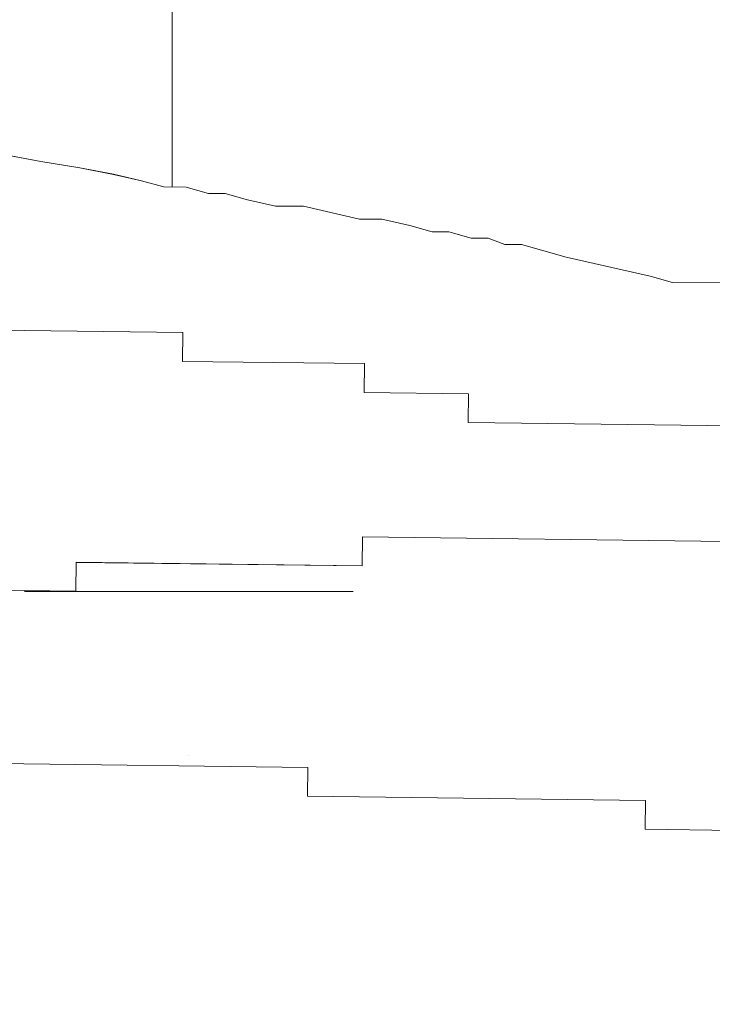
# Model space of a CAD drawing. Units: inches. Extents: x -466983 to 1020, y 324 to 318697.
# Tile 81 of 97: x 656.235 to 659.546, y 944.006 to 948.713. Entities that reach past the tile are written whole.
import ezdxf

# ---------------------------------------------------------------- set-up
doc = ezdxf.new("R2010")
doc.units = ezdxf.units.IN
doc.header["$MEASUREMENT"] = 0
doc.layers.add('A-FLOR-PATT', color=252, linetype='Continuous', lineweight=13)
doc.layers.add('A-FURN', color=8, linetype='Continuous', lineweight=18)

# ---------------------------------------------------------------- blocks, each defined once
blk = doc.blocks.new('L Shaped Sofa')
at = {"ltscale": 2}
for p, q in [((2389.455, 739.834), (2390.5892, 739.8201)), ((2390.5892, 739.8201), (2390.5861, 739.5682)), ((2390.5861, 739.5682), (2393.535, 739.5322)), ((2393.535, 739.5322), (2393.5319, 739.2803)), ((2393.5319, 739.2803), (2396.4808, 739.2443)), ((2394.5686, 739.1785), (2394.5686, 739.1785)), ((2396.0014, 737.7457), (2393.1358, 737.7457)), ((2395.5519, 737.492), (2395.555, 737.7439)), ((2395.555, 737.7439), (2399.8649, 737.6912)), ((2393.0536, 737.2705), (2393.0567, 737.5224)), ((2393.0567, 737.5224), (2395.5519, 737.492)), ((2389.8779, 737.3093), (2393.0536, 737.2705)), ((2386.9167, 736.3377), (2392.134, 736.274)), ((2392.134, 736.274), (2392.1309, 736.0221)), ((2392.1309, 736.0221), (2393.0382, 736.011)), ((2393.0382, 736.011), (2393.0352, 735.7591)), ((2393.0352, 735.7591), (2394.623, 735.7397)), ((2394.623, 735.7397), (2394.6199, 735.4878)), ((2394.6199, 735.4878), (2397.1151, 735.4573)), ((2387.7166, 735.0656), (2390.3515, 735.0532)), ((2390.3515, 735.0532), (2390.5464, 734.9981)), ((2390.5464, 734.9981), (2391.2773, 734.832)), ((2391.2773, 734.832), (2391.667, 734.7217)), ((2391.667, 734.7217), (2391.8134, 734.7211)), ((2391.8134, 734.7211), (2391.9595, 734.6662)), ((2391.9595, 734.6662), (2392.1058, 734.6655)), ((2392.1058, 734.6655), (2392.3007, 734.6103)), ((2392.3007, 734.6103), (2392.4471, 734.6096)), ((2392.4471, 734.6096), (2392.6419, 734.5545)), ((2392.6419, 734.5545), (2392.8856, 734.4992)), ((2392.8856, 734.4992), (2393.0807, 734.4982)), ((2393.0807, 734.4982), (2393.568, 734.3875)), ((2393.568, 734.3875), (2393.812, 734.3864)), ((2393.812, 734.3864), (2394.0556, 734.331)), ((2394.0556, 734.331), (2394.2505, 734.2759)), ((2394.2505, 734.2759), (2394.3969, 734.2752)), ((2394.3969, 734.2752), (2394.5917, 734.2201)), ((2394.5917, 734.2201), (2394.7869, 734.2191)), ((2394.7123, 728.35), (2394.7123, 734.2195)), ((2394.7869, 734.2191), (2394.9818, 734.164)), ((2394.9818, 734.164), (2395.2254, 734.1087)), ((2395.2254, 734.1087), (2395.5178, 734.0531)), ((2395.5178, 734.0531), (2395.8591, 733.9972)), ((2395.8591, 733.9972), (2396.444, 733.8861))]:
    blk.add_line(p, q, dxfattribs=at)

msp = doc.modelspace()

# ---------------------------------------------------------------- hatches: boundary and pattern name
at = {"layer": 'A-FLOR-PATT', "transparency": 33554572}
h = msp.add_hatch(dxfattribs=at)
h.set_pattern_fill('ANSI37', color=256, scale=30)
h.set_pattern_definition([(45, (-1212.4137, -290.035), (-2.6516504, 2.6516504), []), (135, (-1212.4137, -290.035), (-2.6516504, -2.6516504), [])])
h.paths.add_polyline_path([(901.8057, 1075.9377), (900.6144, 1075.9377), (900.6144, 1065.3856), (899.391, 1065.3856), (898.0911, 1065.3856), (892.8356, 1058.7098, -0.258377), (892.1875, 1058.3509), (879.9848, 1058.3509, -0.20177), (879.4382, 1058.5808), (874.0812, 1065.3856), (872.7813, 1065.3856), (871.5579, 1065.3856), (871.5579, 1075.9377), (813.8057, 1075.9377), (813.8057, 1044.7922), (832.3947, 1044.7922, -0.394795), (848.6602, 1028.5356), (848.6602, 1009.9377), (901.8057, 1009.9377), (901.8057, 1015.9377), (901.3057, 1015.9377), (871.3057, 1015.9377), (871.3057, 1017.2502), (871.3344, 1017.2502, -0.401453), (901.3057, 1045.9377), (901.8057, 1045.9377)])
edge = h.paths.add_edge_path(flags=16)
edge.add_line((847.7731, 1068.9486), (847.7731, 1073.7088))
edge.add_arc((849.2269, 1073.7088), 1.4538, 90, 180, ccw=False)
edge.add_line((849.2269, 1075.1627), (864.4921, 1075.1627))
edge.add_arc((864.4921, 1073.7088), 1.4538, 0, 90, ccw=False)
edge.add_line((865.9459, 1073.7088), (865.9459, 1069.0035))
edge.add_arc((832.6447, 1068.9761), 33.3012, -20.61234, 0.04725, ccw=False)
edge.add_ellipse((856.8595, 1058.48), major_axis=(0, 10.2131), ratio=0.6859192, start_angle=100.00884, end_angle=259.99116, ccw=False)
edge.add_arc((881.0742, 1068.9761), 33.3012, 180.04725, 200.61234, ccw=False)
h.paths.add_polyline_path([(853.1456, 1066.4815), (853.1456, 1066.4534), (853.1463, 1066.4534, 0.433107), (852.9166, 1066.6849), (852.9166, 1066.4534), (853.1456, 1066.4534), (853.1456, 1066.4815), (853.088, 1066.6122, 0.697939), (852.6995, 1066.4534), (852.7003, 1066.4534), (852.7003, 1066.4815), (852.9166, 1067.0012), (852.9166, 1066.6849, -0.396254)], flags=0)
h.paths.add_polyline_path([(861.0187, 1066.4815), (861.0187, 1066.4534), (861.0194, 1066.4534, 0.416404), (860.8024, 1066.6849), (860.8024, 1066.4534), (861.0187, 1066.4534), (861.0187, 1066.4815), (860.9672, 1066.6053, 0.713344), (860.5726, 1066.4534), (860.5734, 1066.4534), (860.5734, 1066.4815), (860.8024, 1067.0012), (860.8024, 1066.6849, -0.379973)], flags=0)
edge = h.paths.add_edge_path(flags=0)
edge.add_spline(control_points=[(861.1298, 1065.7855), (861.4661, 1065.2478), (861.6134, 1065.0161), (861.9833, 1064.3736), (862.1924, 1063.9443), (862.5614, 1063.0391), (862.7212, 1062.5633), (862.9865, 1061.5781), (863.092, 1061.0689), (863.2452, 1060.031), (863.293, 1059.5025), (863.3295, 1058.4409), (863.3181, 1057.9078), (863.2366, 1056.8518), (863.1664, 1056.3289), (862.9695, 1055.308), (862.8427, 1054.8099), (862.5365, 1053.8522), (862.3571, 1053.3927), (861.9514, 1052.5249), (861.7251, 1052.1166), (861.233, 1051.3622), (860.9672, 1051.0162), (860.4048, 1050.3949), (860.1082, 1050.1197), (859.4937, 1049.6461), (859.1758, 1049.4476), (858.5276, 1049.1299), (858.1973, 1049.0107), (857.5315, 1048.8518), (857.1959, 1048.8121), (856.5249, 1048.812), (856.1894, 1048.8515), (855.5236, 1049.0101), (855.1933, 1049.1291), (854.545, 1049.4465), (854.2271, 1049.6449), (853.6124, 1050.1183), (853.3158, 1050.3933), (852.7533, 1051.0143), (852.4874, 1051.3602), (851.9952, 1052.1144), (851.7688, 1052.5225), (851.3629, 1053.3902), (851.1834, 1053.8496), (850.877, 1054.8071), (850.7501, 1055.3051), (850.553, 1056.326), (850.4827, 1056.8488), (850.401, 1057.9048), (850.3895, 1058.4379), (850.4257, 1059.4995), (850.4734, 1060.0281), (850.6265, 1061.066), (850.7318, 1061.5753), (850.9969, 1062.5605), (851.1567, 1063.0365), (851.5254, 1063.9418), (851.7345, 1064.3712), (852.1056, 1065.0164), (852.2544, 1065.2503), (852.6082, 1065.7335)], knot_values=[3.915332, 3.915332, 3.915332, 3.915332, 4.013468, 4.013468, 4.175532, 4.175532, 4.337596, 4.337596, 4.49966, 4.49966, 4.661724, 4.661724, 4.823788, 4.823788, 4.985852, 4.985852, 5.147916, 5.147916, 5.30998, 5.30998, 5.472044, 5.472044, 5.634109, 5.634109, 5.796173, 5.796173, 5.958237, 5.958237, 6.120301, 6.120301, 6.282365, 6.282365, 6.444429, 6.444429, 6.606493, 6.606493, 6.768557, 6.768557, 6.930621, 6.930621, 7.092685, 7.092685, 7.254749, 7.254749, 7.416813, 7.416813, 7.578878, 7.578878, 7.740942, 7.740942, 7.903006, 7.903006, 8.06507, 8.06507, 8.227134, 8.227134, 8.389198, 8.389198, 8.551262, 8.551262, 8.65037, 8.65037, 8.65037, 8.65037], degree=3, periodic=0)
edge.add_line((852.6421, 1065.7855), (861.1298, 1065.7855))
edge = h.paths.add_edge_path(flags=0)
edge.add_ellipse((856.8496, 1057.7432), major_axis=(0, 7.7921), ratio=0.687861, start_angle=0, end_angle=360)
h.paths.add_polyline_path([(848.8634, 1069.3891), (848.8634, 1073.9605, -0.414214), (849.9538, 1075.0508), (863.7652, 1075.0508, -0.414214), (864.8555, 1073.9605), (864.8555, 1069.3891, -0.388936), (864.5237, 1069.027, -0.043561), (849.1953, 1069.027, -0.388936)], flags=0)
h.paths.add_polyline_path([(853.1006, 1068.1122, -1), (852.6775, 1068.1122, -1)], flags=0)
edge = h.paths.add_edge_path(flags=0)
edge.add_ellipse((856.8595, 1057.3378), major_axis=(0, 2.207), ratio=0.657164, start_angle=0, end_angle=360)
h.paths.add_polyline_path([(861.0415, 1068.1122, -1), (860.6184, 1068.1122, -1)], flags=0)
edge = h.paths.add_edge_path()
edge.add_line((573.9537, 1057.3412), (573.9537, 1075.9377))
edge.add_line((573.9537, 1075.9377), (558.7308, 1075.9377))
edge.add_line((558.7308, 1075.9377), (558.7308, 1065.3856))
edge.add_line((558.7308, 1065.3856), (557.5074, 1065.3856))
edge.add_line((557.5074, 1065.3856), (556.2075, 1065.3856))
edge.add_line((556.2075, 1065.3856), (550.952, 1058.7098))
edge.add_arc((550.3039, 1059.1155), 0.7646, 270, 327.9483, ccw=False)
edge.add_line((550.3039, 1058.3509), (538.1012, 1058.3509))
edge.add_arc((538.1012, 1059.1155), 0.7646, 224.3704, 270, ccw=False)
edge.add_line((537.5546, 1058.5808), (532.1976, 1065.3856))
edge.add_line((532.1976, 1065.3856), (530.8977, 1065.3856))
edge.add_line((530.8977, 1065.3856), (529.6743, 1065.3856))
edge.add_line((529.6743, 1065.3856), (529.6743, 1075.9377))
edge.add_line((529.6743, 1075.9377), (520.8057, 1075.9377))
edge.add_line((520.8057, 1075.9377), (520.8057, 1045.9377))
edge.add_line((520.8057, 1045.9377), (521.3057, 1045.9377))
edge.add_arc((521.3057, 1015.9377), 30, 2.50749, 90, ccw=False)
edge.add_line((551.277, 1017.2502), (551.3057, 1017.2502))
edge.add_line((551.3057, 1017.2502), (551.3057, 1015.9377))
edge.add_line((551.3057, 1015.9377), (520.8057, 1015.9377))
edge.add_line((520.8057, 1015.9377), (520.8057, 1009.9377))
edge.add_line((520.8057, 1009.9377), (559.1913, 1010.4022))
edge.add_arc((559.1913, 1011.856), 1.4538, 180, 270, ccw=False)
edge.add_line((557.7375, 1011.856), (557.7375, 1016.5613))
edge.add_arc((591.0386, 1016.5888), 33.3012, 159.38766, 180.04725, ccw=False)
edge.add_ellipse((566.8239, 1027.0848), major_axis=(0, 10.2131), ratio=0.6859192, start_angle=280.00884, end_angle=439.99116, ccw=False)
edge.add_arc((542.6091, 1016.5888), 33.3012, 0.04725, 20.61234, ccw=False)
edge.add_line((575.9103, 1016.6162), (575.9103, 1011.856))
edge.add_arc((574.4565, 1011.856), 1.4538, -90, 0, ccw=False)
edge.add_line((574.4565, 1010.4022), (608.8057, 1009.9377))
edge.add_line((608.8057, 1009.9377), (608.8057, 1041.0857))
edge.add_line((608.8057, 1041.0857), (590.2179, 1041.0857))
edge.add_arc((590.775, 1057.9074), 16.8309, 181.92775, 268.10321, ccw=False)
edge = h.paths.add_edge_path()
edge.add_ellipse((494.2443, 583.6204), major_axis=(0, 10.2131), ratio=0.6859192, start_angle=280.00884, end_angle=439.99116, ccw=False)
edge.add_arc((470.0296, 573.1243), 33.3012, 0.04725, 20.61234, ccw=False)
edge.add_line((503.3307, 573.1518), (503.3307, 568.3916))
edge.add_arc((501.8769, 568.3916), 1.4538, -90, 0, ccw=False)
edge.add_line((501.8769, 566.9377), (539.8057, 566.9377))
edge.add_line((539.8057, 566.9377), (539.8057, 572.9377))
edge.add_line((539.8057, 572.9377), (539.3057, 572.9377))
edge.add_line((539.3057, 572.9377), (509.3057, 572.9377))
edge.add_line((509.3057, 572.9377), (509.3057, 574.2502))
edge.add_line((509.3057, 574.2502), (509.3344, 574.2502))
edge.add_arc((539.3057, 572.9377), 30, 90, 177.49251, ccw=False)
edge.add_line((539.3057, 602.9377), (539.8057, 602.9377))
edge.add_line((539.8057, 602.9377), (539.8057, 626.9377))
edge.add_line((539.8057, 626.9377), (531.7718, 626.9377))
edge.add_line((531.7718, 626.9377), (531.7718, 616.3856))
edge.add_line((531.7718, 616.3856), (530.5484, 616.3856))
edge.add_line((530.5484, 616.3856), (529.2485, 616.3856))
edge.add_line((529.2485, 616.3856), (523.7105, 609.3509))
edge.add_line((523.7105, 609.3509), (510.7766, 609.3509))
edge.add_line((510.7766, 609.3509), (505.2386, 616.3856))
edge.add_line((505.2386, 616.3856), (503.9387, 616.3856))
edge.add_line((503.9387, 616.3856), (502.7153, 616.3856))
edge.add_line((502.7153, 616.3856), (502.7153, 626.9377))
edge.add_line((502.7153, 626.9377), (481.6983, 626.9377))
edge.add_line((481.6983, 626.9377), (481.6983, 610.995))
edge.add_arc((467.2703, 611.4728), 14.4359, 271.92775, 358.10321, ccw=False)
edge.add_line((467.7559, 597.0451), (451.8057, 597.0451))
edge.add_line((451.8057, 597.0451), (451.8057, 584.4035))
edge.add_line((451.8057, 584.4035), (451.8057, 566.9377))
edge.add_line((451.8057, 566.9377), (486.6117, 566.9377))
edge.add_arc((486.6117, 568.3916), 1.4538, 180, 270, ccw=False)
edge.add_line((485.1579, 568.3916), (485.1579, 573.0969))
edge.add_arc((518.4591, 573.1243), 33.3012, 159.38766, 180.04725, ccw=False)
h.paths.add_polyline_path([(836.2609, 1020.7328), (879.8898, 1020.7328), (879.8898, 1039.3902), (836.2609, 1039.3902)], flags=25)
h.paths.add_polyline_path([(549.9851, 1036.7492), (593.614, 1036.7492), (593.614, 1055.4065), (549.9851, 1055.4065)], flags=24)
h.paths.add_polyline_path([(475.123, 595.5959), (518.752, 595.5959), (518.752, 614.2532), (475.123, 614.2532)], flags=24)
h = msp.add_hatch(dxfattribs=at)
h.set_pattern_fill('ANSI37', color=256, scale=20)
h.set_pattern_definition([(45, (-1212.4137, -290.035), (-1.767767, 1.767767), []), (135, (-1212.4137, -290.035), (-1.767767, -1.767767), [])])
h.paths.add_polyline_path([(809.8057, 870.9377), (809.8057, 888.1519), (806.9985, 888.1519), (802.6624, 888.1519), (789.3832, 888.1519), (786.2846, 888.1519, -0.414214), (785.4991, 888.9374), (785.4991, 900.1959), (785.4991, 908.4696, -0.414214), (786.8082, 909.7787, -0.414214), (785.4991, 911.0878), (785.4991, 929.1015, -0.414214), (786.8082, 930.4106, -0.414214), (785.4991, 931.7197), (785.4991, 931.9039, -0.414214), (784.19, 930.5948), (766.7223, 930.5948, -0.412359), (765.4132, 931.8956, -0.413741), (764.1145, 930.5782), (744.5781, 930.422, -0.416556), (743.7864, 931.2075), (743.7864, 933.5153), (742.2154, 933.5153), (742.2154, 952.024, -0.001344), (743.7864, 952.1998), (743.7864, 953.9377), (678.5915, 953.9377), (678.5915, 951.1305), (678.5915, 946.7945), (678.5915, 933.5153), (678.5915, 930.4166, -0.414214), (677.806, 929.6312), (666.5475, 929.6312), (658.2738, 929.6312, -0.414214), (656.9647, 930.9403, -0.414214), (655.6556, 929.6312), (637.6419, 929.6312, -0.414214), (636.3328, 930.9403, -0.414214), (635.0237, 929.6312), (634.8395, 929.6312, -0.414214), (636.1486, 928.322), (636.1486, 910.8544, -0.412359), (634.8478, 909.5452, -0.413741), (636.1653, 908.2466), (636.3214, 888.7102, -0.416556), (635.5359, 887.9184), (633.2281, 887.9184), (633.2281, 886.3475), (614.7194, 886.3475, -0.001344), (614.5436, 887.9184), (612.8057, 887.9184), (612.8057, 834.9377), (612.8057, 752.9377), (612.8057, 748.9377), (612.8057, 697.9377), (654.8057, 697.9377), (654.8057, 701.9377), (715.8057, 701.9377), (715.8057, 737.4353), (774.2918, 737.4353), (774.2918, 795.9377), (809.8057, 795.9377)])
h.paths.add_polyline_path([(679.2761, 849.5757, 0.102523), (682.1475, 849.2608, -0.080461), (694.5428, 849.7725, -0.283899), (694.4822, 849.0082, 0.136605), (694.4068, 848.8103, -0.030441), (694.5428, 846.8929), (694.5428, 842.6198), (694.5428, 838.3466, -0.028219), (694.4246, 836.5684), (694.425, 836.5684, 0.196187), (694.4456, 836.2708, -0.302897), (694.5428, 835.467, -0.080461), (682.1475, 835.9787, 0.102523), (679.2761, 835.6638, -0.58611), (678.6457, 836.0169), (678.6457, 849.2227, -0.58611)], flags=16)
h.paths.add_polyline_path([(679.5173, 848.6515, 0.699597), (679.476, 848.6342, 1.20716), (679.1935, 848.7422, 0.010621)], flags=0)
h.paths.add_polyline_path([(679.4923, 836.5608, -0.013798), (679.9178, 836.6594, -0.071703), (682.8533, 837.1434, -0.165743), (682.1665, 839.1006), (682.1665, 842.6094), (682.1665, 846.0603, -0.240616), (683.4733, 848.6767, -0.068263), (693.9295, 849.0082), (693.7875, 848.7083), (693.7875, 849.0228, 0.067332), (683.4733, 848.6767, 0.240616), (682.1665, 846.0603), (682.1665, 842.6094), (682.1665, 839.1006, 0.23459), (683.461, 836.5513, 0.068093), (693.7875, 836.1955), (693.7875, 836.5104), (693.9296, 836.2102, -0.077215), (682.2421, 836.7815, 0.086627), (679.5283, 836.5701, -0.628402), (679.5029, 836.5735), (679.5029, 836.6071, 0.910458)], flags=0)
h.paths.add_polyline_path([(679.476, 848.6364), (679.2069, 848.647), (679.2069, 836.5718, 0.913566), (679.3645, 836.5861), (679.476, 836.5824)], flags=0)
h.paths.add_polyline_path([(679.2761, 829.8604, 0.102523), (682.1475, 829.5455, -0.080461), (694.5428, 830.0572, -0.283899), (694.4822, 829.2929, 0.136605), (694.4068, 829.095, -0.030441), (694.5428, 827.1776), (694.5428, 822.9045), (694.5428, 818.6314, -0.028219), (694.4246, 816.8531), (694.425, 816.8532, 0.196187), (694.4456, 816.5555, -0.302897), (694.5428, 815.7517, -0.080461), (682.1475, 816.2635, 0.102523), (679.2761, 815.9485, -0.58611), (678.6457, 816.3016), (678.6457, 829.5074, -0.58611)], flags=16)
h.paths.add_polyline_path([(679.5173, 828.9362, 0.699597), (679.476, 828.9189, 1.20716), (679.1935, 829.0269, 0.010621)], flags=0)
h.paths.add_polyline_path([(679.4923, 816.8456, -0.013798), (679.9178, 816.9441, -0.071703), (682.8533, 817.4281, -0.165743), (682.1665, 819.3853), (682.1665, 822.8941), (682.1665, 826.345, -0.240616), (683.4733, 828.9614, -0.068263), (693.9295, 829.2929), (693.7875, 828.9931), (693.7875, 829.3076, 0.067332), (683.4733, 828.9614, 0.240616), (682.1665, 826.345), (682.1665, 822.8941), (682.1665, 819.3853, 0.23459), (683.461, 816.836, 0.068093), (693.7875, 816.4802), (693.7875, 816.7952), (693.9296, 816.4949, -0.077215), (682.2421, 817.0662, 0.086627), (679.5283, 816.8549, -0.628402), (679.5029, 816.8582), (679.5029, 816.8918, 0.910458)], flags=0)
h.paths.add_polyline_path([(679.476, 828.9211), (679.2069, 828.9317), (679.2069, 816.8565, 0.913566), (679.3645, 816.8708), (679.476, 816.8671)], flags=0)
h.paths.add_polyline_path([(679.2761, 810.1451, 0.102523), (682.1475, 809.8302, -0.080461), (694.5428, 810.342, -0.3023), (694.4466, 809.5394, 0.10023), (694.4058, 809.3878, -0.03057), (694.5428, 807.4623), (694.5428, 803.1892), (694.5428, 798.9161, -0.03057), (694.4058, 796.9906, 0.10023), (694.4466, 796.839, -0.3023), (694.5428, 796.0365, -0.080461), (682.1475, 796.5482, 0.102523), (679.2761, 796.2333, -0.58611), (678.6457, 796.5863), (678.6457, 809.7921, -0.58611)], flags=16)
h.paths.add_polyline_path([(679.5173, 809.2417, 0.699597), (679.476, 809.2244, 1.20716), (679.1935, 809.3324, 0.010621)], flags=0)
h.paths.add_polyline_path([(679.4923, 797.151, -0.013798), (679.9178, 797.2496, -0.071703), (682.8533, 797.7336, -0.165743), (682.1665, 799.6908), (682.1665, 803.1996), (682.1665, 806.6505, -0.239349), (683.461, 809.2577, -0.072465), (694.4468, 809.5405, 0.197932), (694.425, 809.2405), (693.7875, 809.2985), (693.7875, 809.6135, 0.068093), (683.461, 809.2577, 0.239349), (682.1665, 806.6505), (682.1665, 803.1996), (682.1665, 799.6908, 0.235854), (683.4733, 797.1323, 0.067332), (693.7875, 796.7861), (693.7875, 797.1006), (694.425, 797.1586, 0.197932), (694.4468, 796.8586, -0.080419), (682.1557, 797.3795, 0.083867), (679.5283, 797.1603, -0.628402), (679.5029, 797.1637), (679.5029, 797.1973, 0.910458)], flags=0)
h.paths.add_polyline_path([(679.2069, 809.2372), (679.2069, 797.162, 0.913566), (679.3645, 797.1763), (679.476, 797.1726), (679.476, 809.2266)], flags=0)
h.paths.add_polyline_path([(695.3643, 853.2989), (728.2231, 853.2989), (728.2231, 771.1519), (695.3643, 771.1519)], flags=16)
h.paths.add_polyline_path([(696.0215, 852.6417), (727.5659, 852.6417), (727.5659, 771.809), (696.0215, 771.809)], flags=0)
h.paths.add_polyline_path([(679.2761, 788.7869, 0.102523), (682.1475, 788.472, -0.080461), (694.5428, 788.9837, -0.3023), (694.4466, 788.1812, 0.10023), (694.4058, 788.0296, -0.03057), (694.5428, 786.1041), (694.5428, 781.831), (694.5428, 777.5578, -0.03057), (694.4058, 775.6323, 0.10023), (694.4466, 775.4808, -0.3023), (694.5428, 774.6782, -0.080461), (682.1475, 775.19, 0.102523), (679.2761, 774.875, -0.58611), (678.6457, 775.2281), (678.6457, 788.4339, -0.58611)], flags=16)
h.paths.add_polyline_path([(679.5173, 787.8834, 0.699597), (679.476, 787.8662, 1.20716), (679.1935, 787.9742, 0.010621)], flags=0)
h.paths.add_polyline_path([(679.4923, 775.7928, -0.013798), (679.9178, 775.8914, -0.071703), (682.8533, 776.3753, -0.165743), (682.1665, 778.3325), (682.1665, 781.8414), (682.1665, 785.2922, -0.239349), (683.461, 787.8995, -0.072465), (694.4468, 788.1823, 0.197932), (694.425, 787.8823), (693.7875, 787.9403), (693.7875, 788.2553, 0.068093), (683.461, 787.8995, 0.239349), (682.1665, 785.2922), (682.1665, 781.8414), (682.1665, 778.3325, 0.235854), (683.4733, 775.7741, 0.067332), (693.7875, 775.4279), (693.7875, 775.7424), (694.425, 775.8004, 0.197932), (694.4468, 775.5004, -0.080419), (682.1557, 776.0212, 0.083867), (679.5283, 775.8021, -0.628402), (679.5029, 775.8054), (679.5029, 775.8391, 0.910458)], flags=0)
h.paths.add_polyline_path([(679.2069, 787.8789), (679.2069, 775.8038, 0.913566), (679.3645, 775.818), (679.476, 775.8144), (679.476, 787.8684)], flags=0)
h.paths.add_polyline_path([(704.641, 854.1204, -0.080461), (705.1527, 866.5157, 0.102523), (704.8378, 869.3871, -0.58611), (705.1908, 870.0174), (718.3966, 870.0174, -0.58611), (718.7496, 869.3871, 0.102523), (718.4347, 866.5157, -0.080461), (718.9465, 854.1204, -0.3023), (718.1439, 854.2166, 0.10023), (717.9924, 854.2574, -0.03057), (716.0668, 854.1204), (711.7937, 854.1204), (707.5206, 854.1204, -0.03057), (705.5951, 854.2574, 0.10023), (705.4435, 854.2166, -0.3023)], flags=16)
h.paths.add_polyline_path([(717.8462, 869.1459, 0.699597), (717.8289, 869.1872, 1.20716), (717.9369, 869.4697, 0.010621)], flags=0)
h.paths.add_polyline_path([(705.4631, 854.2164, -0.080419), (705.984, 866.5074, 0.083867), (705.7648, 869.1349, -0.628402), (705.7682, 869.1603), (705.8018, 869.1603, 0.910458), (705.7555, 869.1709, -0.013798), (705.8541, 868.7454, -0.071703), (706.3381, 865.8099, -0.165743), (708.2953, 866.4967), (711.8041, 866.4967), (715.255, 866.4967, -0.239349), (717.8622, 865.2022, -0.072465), (718.145, 854.2164, 0.197932), (717.845, 854.2382), (717.903, 854.8757), (718.218, 854.8757, 0.068093), (717.8622, 865.2022, 0.239349), (715.255, 866.4967), (711.8041, 866.4967), (708.2953, 866.4967, 0.235854), (705.7368, 865.1898, 0.067332), (705.3906, 854.8757), (705.7051, 854.8757), (705.7631, 854.2382, 0.197932)], flags=16)
h.paths.add_polyline_path([(705.7665, 869.4563, 0.913566), (705.7808, 869.2987), (705.7771, 869.1872), (717.8311, 869.1872), (717.8417, 869.4563)], flags=0)
h.paths.add_polyline_path([(729.0446, 842.6198), (729.0446, 846.8929, -0.03057), (729.1817, 848.8184, 0.10023), (729.1408, 848.9699, -0.3023), (729.0446, 849.7725, -0.080461), (741.4399, 849.2608, 0.102523), (744.3113, 849.5757, -0.58611), (744.9417, 849.2227), (744.9417, 836.0169, -0.58611), (744.3113, 835.6638, 0.102523), (741.4399, 835.9787, -0.080461), (729.0446, 835.467, -0.3023), (729.1408, 836.2696, 0.10023), (729.1817, 836.4211, -0.03057), (729.0446, 838.3466)], flags=16)
h.paths.add_polyline_path([(744.1115, 836.5846, 1.20716), (744.3939, 836.4766, 0.010621), (744.0701, 836.5673, 0.699597)], flags=0)
h.paths.add_polyline_path([(729.1407, 836.2684, 0.197932), (729.1624, 836.5684), (729.7999, 836.5104), (729.7999, 836.1955, 0.068093), (740.1264, 836.5513, 0.239349), (741.4209, 839.1585), (741.4209, 842.6094), (741.4209, 846.1182, 0.235854), (740.1141, 848.6767, 0.067332), (729.7999, 849.0228), (729.7999, 848.7083), (729.1624, 848.6503, 0.197932), (729.1407, 848.9504, -0.080419), (741.4317, 848.4295, 0.083867), (744.0591, 848.6486, -0.628402), (744.0845, 848.6453), (744.0845, 848.6117, 0.910458), (744.0951, 848.6579, -0.013798), (743.6696, 848.5594, -0.071703), (740.7341, 848.0754, -0.165743), (741.4209, 846.1182), (741.4209, 842.6094), (741.4209, 839.1585, -0.239349), (740.1264, 836.5513, -0.072465)], flags=0)
h.paths.add_polyline_path([(729.0446, 830.0572, -0.080461), (741.4399, 829.5455, 0.102523), (744.3113, 829.8604, -0.58611), (744.9417, 829.5074), (744.9417, 816.3016, -0.58611), (744.3113, 815.9485, 0.102523), (741.4399, 816.2635, -0.080461), (729.0446, 815.7517, -0.3023), (729.1408, 816.5543, 0.10023), (729.1817, 816.7058, -0.03057), (729.0446, 818.6314), (729.0446, 822.9045), (729.0446, 827.1776, -0.03057), (729.1817, 829.1031, 0.10023), (729.1408, 829.2547, -0.3023)], flags=16)
h.paths.add_polyline_path([(744.1115, 816.8693, 1.20716), (744.3939, 816.7613, 0.010621), (744.0701, 816.852, 0.699597)], flags=0)
h.paths.add_polyline_path([(729.1407, 829.2351, -0.080419), (741.4317, 828.7142, 0.083867), (744.0591, 828.9334, -0.628402), (744.0845, 828.93), (744.0845, 828.8964, 0.910458), (744.0951, 828.9427, -0.013798), (743.6696, 828.8441, -0.071703), (740.7341, 828.3601, -0.165743), (741.4209, 826.4029), (741.4209, 822.8941), (741.4209, 819.4432, -0.239349), (740.1264, 816.836, -0.072465), (729.1407, 816.5531, 0.197932), (729.1624, 816.8532), (729.7999, 816.7952), (729.7999, 816.4802, 0.068093), (740.1264, 816.836, 0.239349), (741.4209, 819.4432), (741.4209, 822.8941), (741.4209, 826.4029, 0.235854), (740.1141, 828.9614, 0.067332), (729.7999, 829.3076), (729.7999, 828.9931), (729.1624, 828.9351, 0.197932)], flags=16)
h.paths.add_polyline_path([(729.0446, 810.342, -0.080461), (741.4399, 809.8302, 0.102523), (744.3113, 810.1451, -0.58611), (744.9417, 809.7921), (744.9417, 796.5863, -0.58611), (744.3113, 796.2333, 0.102523), (741.4399, 796.5482, -0.080461), (729.0446, 796.0365, -0.283899), (729.1052, 796.8007, 0.136605), (729.1806, 796.9987, -0.030441), (729.0446, 798.9161), (729.0446, 803.1892), (729.0446, 807.4623, -0.028219), (729.1628, 809.2406), (729.1624, 809.2405, 0.196187), (729.1418, 809.5382, -0.302897)], flags=16)
h.paths.add_polyline_path([(744.1115, 797.1748, 1.20716), (744.3939, 797.0668, 0.010621), (744.0701, 797.1575, 0.699597)], flags=0)
h.paths.add_polyline_path([(741.3453, 809.0275, 0.086627), (744.0591, 809.2388, -0.628402), (744.0845, 809.2355), (744.0845, 809.2019, 0.910458), (744.0951, 809.2481, -0.013798), (743.6696, 809.1496, -0.071703), (740.7341, 808.6656, -0.165743), (741.4209, 806.7084), (741.4209, 803.1996), (741.4209, 799.7487, -0.240616), (740.1141, 797.1323, -0.068263), (729.658, 796.8008), (729.7999, 797.1006), (729.7999, 796.7861, 0.067332), (740.1141, 797.1323, 0.240616), (741.4209, 799.7487), (741.4209, 803.1996), (741.4209, 806.7084, 0.23459), (740.1264, 809.2577, 0.068093), (729.7999, 809.6135), (729.7999, 809.2985), (729.6578, 809.5988, -0.077215)], flags=0)
h.paths.add_polyline_path([(704.641, 770.3304, -0.283899), (705.4053, 770.2697, 0.136605), (705.6032, 770.1944, -0.030441), (707.5206, 770.3304), (711.7937, 770.3304), (716.0668, 770.3304, -0.028219), (717.8451, 770.2122), (717.845, 770.2126, 0.196187), (718.1427, 770.2331, -0.302897), (718.9465, 770.3304, -0.080461), (718.4347, 757.9351, 0.102523), (718.7496, 755.0637, -0.58611), (718.3966, 754.4333), (705.1908, 754.4333, -0.58611), (704.8378, 755.0637, 0.102523), (705.1527, 757.9351, -0.080461)], flags=16)
h.paths.add_polyline_path([(705.762, 755.3048, 0.699597), (705.7793, 755.2635, 1.20716), (705.6713, 754.9811, 0.010621)], flags=0)
h.paths.add_polyline_path([(705.4053, 769.717), (705.7051, 769.5751), (705.3906, 769.5751, 0.067332), (705.7368, 759.2609, 0.240616), (708.3532, 757.954), (711.8041, 757.954), (715.3129, 757.954, 0.23459), (717.8622, 759.2485, 0.068093), (718.218, 769.5751), (717.903, 769.5751), (718.2033, 769.7172, -0.077215), (717.632, 758.0297, 0.086627), (717.8433, 755.3159, -0.628402), (717.84, 755.2904), (717.8064, 755.2904, 0.910458), (717.8526, 755.2799, -0.013798), (717.7541, 755.7053, -0.071703), (717.2701, 758.6409, -0.165743), (715.3129, 757.954), (711.8041, 757.954), (708.3532, 757.954, -0.240616), (705.7368, 759.2609, -0.068263)], flags=0)
h.paths.add_polyline_path([(729.0446, 788.9837, -0.080461), (741.4399, 788.472, 0.102523), (744.3113, 788.7869, -0.58611), (744.9417, 788.4339), (744.9417, 775.2281, -0.58611), (744.3113, 774.875, 0.102523), (741.4399, 775.19, -0.080461), (729.0446, 774.6782, -0.283899), (729.1052, 775.4425, 0.136605), (729.1806, 775.6405, -0.030441), (729.0446, 777.5578), (729.0446, 781.831), (729.0446, 786.1041, -0.028219), (729.1628, 787.8823), (729.1624, 787.8823, 0.196187), (729.1418, 788.1799, -0.302897)], flags=16)
h.paths.add_polyline_path([(744.1115, 775.8165, 1.20716), (744.3939, 775.7086, 0.010621), (744.0701, 775.7993, 0.699597)], flags=0)
h.paths.add_polyline_path([(741.3453, 787.6692, 0.086627), (744.0591, 787.8806, -0.628402), (744.0845, 787.8773), (744.0845, 787.8437, 0.910458), (744.0951, 787.8899, -0.013798), (743.6696, 787.7913, -0.071703), (740.7341, 787.3074, -0.165743), (741.4209, 785.3502), (741.4209, 781.8414), (741.4209, 778.3905, -0.240616), (740.1141, 775.7741, -0.068263), (729.658, 775.4425), (729.7999, 775.7424), (729.7999, 775.4279, 0.067332), (740.1141, 775.7741, 0.240616), (741.4209, 778.3905), (741.4209, 781.8414), (741.4209, 785.3502, 0.23459), (740.1264, 787.8995, 0.068093), (729.7999, 788.2553), (729.7999, 787.9403), (729.6578, 788.2405, -0.077215)], flags=0)
h.paths.add_polyline_path([(744.1115, 848.6364), (744.1115, 836.5824), (744.3805, 836.5718), (744.3805, 848.647, 0.913566), (744.2229, 848.6327)], flags=0)
h.paths.add_polyline_path([(744.2229, 828.9174), (744.1115, 828.9211), (744.1115, 816.8671), (744.3805, 816.8565), (744.3805, 828.9317, 0.913566)], flags=0)
h.paths.add_polyline_path([(717.8311, 755.2635), (705.7771, 755.2635), (705.7665, 754.9945), (717.8417, 754.9945, 0.913566), (717.8274, 755.1521)], flags=0)
h.paths.add_polyline_path([(744.2229, 809.2229), (744.1115, 809.2266), (744.1115, 797.1726), (744.3805, 797.162), (744.3805, 809.2372, 0.913566)], flags=0)
h.paths.add_polyline_path([(744.1115, 787.8684), (744.1115, 775.8144), (744.3805, 775.8038), (744.3805, 787.8789, 0.913566), (744.2229, 787.8647)], flags=0)
h.paths.add_polyline_path([(678.8774, 877.1228), (737.6127, 877.1228), (737.6127, 899.5116), (678.8774, 899.5116)], flags=24)

# ---------------------------------------------------------------- linework, layer by layer
at = {"layer": 'A-FURN', "ltscale": 2}
for p, q in [((656.9647, 951.1305), (656.9647, 947.9128)), ((656.9647, 951.1305), (656.9647, 947.9128)), ((656.9647, 951.1305), (656.9647, 947.9128)), ((656.9647, 951.1305), (656.9647, 947.9128)), ((656.9647, 951.1305), (656.9647, 947.9128)), ((656.9647, 951.1305), (656.9647, 947.9128)), ((656.336, 948.0346), (656.0154, 948.0956)), ((656.336, 948.0346), (656.0154, 948.0956)), ((656.336, 948.0346), (656.0154, 948.0956)), ((656.336, 948.0346), (656.0154, 948.0956)), ((656.336, 948.0346), (656.0154, 948.0956)), ((656.336, 948.0346), (656.0154, 948.0956)), ((656.5231, 948.004), (656.336, 948.0346)), ((656.5231, 948.004), (656.336, 948.0346)), ((656.5231, 948.004), (656.336, 948.0346)), ((656.5231, 948.004), (656.336, 948.0346)), ((656.5231, 948.004), (656.336, 948.0346)), ((656.5231, 948.004), (656.336, 948.0346)), ((656.6834, 947.9736), (656.5231, 948.004)), ((656.6834, 947.9736), (656.5231, 948.004)), ((656.6834, 947.9736), (656.5231, 948.004)), ((656.6834, 947.9736), (656.5231, 948.004)), ((656.6834, 947.9736), (656.5231, 948.004)), ((656.6834, 947.9736), (656.5231, 948.004)), ((656.817, 947.9432), (656.6834, 947.9736)), ((656.817, 947.9432), (656.6834, 947.9736)), ((656.817, 947.9432), (656.6834, 947.9736)), ((656.817, 947.9432), (656.6834, 947.9736)), ((656.817, 947.9432), (656.6834, 947.9736)), ((656.817, 947.9432), (656.6834, 947.9736)), ((656.9238, 947.913), (656.817, 947.9432)), ((656.9238, 947.913), (656.817, 947.9432)), ((656.9238, 947.913), (656.817, 947.9432)), ((656.9238, 947.913), (656.817, 947.9432)), ((656.9238, 947.913), (656.817, 947.9432)), ((656.9238, 947.913), (656.817, 947.9432)), ((657.0308, 947.9125), (656.9238, 947.913)), ((657.0308, 947.9125), (656.9238, 947.913)), ((657.0308, 947.9125), (656.9238, 947.913)), ((657.0308, 947.9125), (656.9238, 947.913)), ((657.0308, 947.9125), (656.9238, 947.913)), ((657.0308, 947.9125), (656.9238, 947.913)), ((657.1376, 947.8823), (657.0308, 947.9125)), ((657.1376, 947.8823), (657.0308, 947.9125)), ((657.1376, 947.8823), (657.0308, 947.9125)), ((657.1376, 947.8823), (657.0308, 947.9125)), ((657.1376, 947.8823), (657.0308, 947.9125)), ((657.1376, 947.8823), (657.0308, 947.9125)), ((657.2179, 947.8819), (657.1376, 947.8823)), ((657.2179, 947.8819), (657.1376, 947.8823)), ((657.2179, 947.8819), (657.1376, 947.8823)), ((657.2179, 947.8819), (657.1376, 947.8823)), ((657.2179, 947.8819), (657.1376, 947.8823)), ((657.2179, 947.8819), (657.1376, 947.8823)), ((657.3247, 947.8517), (657.2179, 947.8819)), ((657.3247, 947.8517), (657.2179, 947.8819)), ((657.3247, 947.8517), (657.2179, 947.8819)), ((657.3247, 947.8517), (657.2179, 947.8819)), ((657.3247, 947.8517), (657.2179, 947.8819)), ((657.3247, 947.8517), (657.2179, 947.8819)), ((657.4583, 947.8213), (657.3247, 947.8517)), ((657.4583, 947.8213), (657.3247, 947.8517)), ((657.4583, 947.8213), (657.3247, 947.8517)), ((657.4583, 947.8213), (657.3247, 947.8517)), ((657.4583, 947.8213), (657.3247, 947.8517)), ((657.4583, 947.8213), (657.3247, 947.8517)), ((657.592, 947.8207), (657.4583, 947.8213)), ((657.592, 947.8207), (657.4583, 947.8213)), ((657.592, 947.8207), (657.4583, 947.8213)), ((657.592, 947.8207), (657.4583, 947.8213)), ((657.592, 947.8207), (657.4583, 947.8213)), ((657.592, 947.8207), (657.4583, 947.8213)), ((657.8591, 947.76), (657.592, 947.8207)), ((657.8591, 947.76), (657.592, 947.8207)), ((657.8591, 947.76), (657.592, 947.8207)), ((657.8591, 947.76), (657.592, 947.8207)), ((657.8591, 947.76), (657.592, 947.8207)), ((657.8591, 947.76), (657.592, 947.8207)), ((657.9661, 947.7595), (657.8591, 947.76)), ((657.9661, 947.7595), (657.8591, 947.76)), ((657.9661, 947.7595), (657.8591, 947.76)), ((657.9661, 947.7595), (657.8591, 947.76)), ((657.9661, 947.7595), (657.8591, 947.76)), ((657.9661, 947.7595), (657.8591, 947.76)), ((658.0997, 947.7291), (657.9661, 947.7595)), ((658.0997, 947.7291), (657.9661, 947.7595)), ((658.0997, 947.7291), (657.9661, 947.7595)), ((658.0997, 947.7291), (657.9661, 947.7595)), ((658.0997, 947.7291), (657.9661, 947.7595)), ((658.0997, 947.7291), (657.9661, 947.7595)), ((658.2065, 947.6989), (658.0997, 947.7291)), ((658.2065, 947.6989), (658.0997, 947.7291)), ((658.2065, 947.6989), (658.0997, 947.7291)), ((658.2065, 947.6989), (658.0997, 947.7291)), ((658.2065, 947.6989), (658.0997, 947.7291)), ((658.2065, 947.6989), (658.0997, 947.7291)), ((658.2868, 947.6985), (658.2065, 947.6989)), ((658.2868, 947.6985), (658.2065, 947.6989)), ((658.2868, 947.6985), (658.2065, 947.6989)), ((658.2868, 947.6985), (658.2065, 947.6989)), ((658.2868, 947.6985), (658.2065, 947.6989)), ((658.2868, 947.6985), (658.2065, 947.6989)), ((658.3936, 947.6683), (658.2868, 947.6985)), ((658.3936, 947.6683), (658.2868, 947.6985)), ((658.3936, 947.6683), (658.2868, 947.6985)), ((658.3936, 947.6683), (658.2868, 947.6985)), ((658.3936, 947.6683), (658.2868, 947.6985)), ((658.3936, 947.6683), (658.2868, 947.6985)), ((658.4739, 947.6679), (658.3936, 947.6683)), ((658.4739, 947.6679), (658.3936, 947.6683)), ((658.4739, 947.6679), (658.3936, 947.6683)), ((658.4739, 947.6679), (658.3936, 947.6683)), ((658.4739, 947.6679), (658.3936, 947.6683)), ((658.4739, 947.6679), (658.3936, 947.6683)), ((658.5539, 947.6378), (658.4739, 947.6679)), ((658.5539, 947.6378), (658.4739, 947.6679)), ((658.5539, 947.6378), (658.4739, 947.6679)), ((658.5539, 947.6378), (658.4739, 947.6679)), ((658.5539, 947.6378), (658.4739, 947.6679)), ((658.5539, 947.6378), (658.4739, 947.6679)), ((658.6342, 947.6375), (658.5539, 947.6378)), ((658.6342, 947.6375), (658.5539, 947.6378)), ((658.6342, 947.6375), (658.5539, 947.6378)), ((658.6342, 947.6375), (658.5539, 947.6378)), ((658.6342, 947.6375), (658.5539, 947.6378)), ((658.6342, 947.6375), (658.5539, 947.6378)), ((658.8478, 947.577), (658.6342, 947.6375)), ((658.8478, 947.577), (658.6342, 947.6375)), ((658.8478, 947.577), (658.6342, 947.6375)), ((658.8478, 947.577), (658.6342, 947.6375)), ((658.8478, 947.577), (658.6342, 947.6375)), ((658.8478, 947.577), (658.6342, 947.6375)), ((659.2485, 947.486), (658.8478, 947.577)), ((659.2485, 947.486), (658.8478, 947.577)), ((659.2485, 947.486), (658.8478, 947.577)), ((659.2485, 947.486), (658.8478, 947.577)), ((659.2485, 947.486), (658.8478, 947.577)), ((659.2485, 947.486), (658.8478, 947.577)), ((659.3553, 947.4557), (659.2485, 947.486)), ((659.3553, 947.4557), (659.2485, 947.486)), ((659.3553, 947.4557), (659.2485, 947.486)), ((659.3553, 947.4557), (659.2485, 947.486)), ((659.3553, 947.4557), (659.2485, 947.486)), ((659.3553, 947.4557), (659.2485, 947.486)), ((660.7999, 947.449), (659.3553, 947.4557)), ((660.7999, 947.449), (659.3553, 947.4557)), ((660.7999, 947.449), (659.3553, 947.4557)), ((660.7999, 947.449), (659.3553, 947.4557)), ((660.7999, 947.449), (659.3553, 947.4557)), ((660.7999, 947.449), (659.3553, 947.4557)), ((657.0153, 947.2175), (655.6474, 947.2342)), ((657.0153, 947.2175), (655.6474, 947.2342)), ((657.0153, 947.2175), (655.6474, 947.2342)), ((657.0153, 947.2175), (655.6474, 947.2342)), ((657.0153, 947.2175), (655.6474, 947.2342)), ((657.0153, 947.2175), (655.6474, 947.2342)), ((657.0137, 947.0794), (657.0153, 947.2175)), ((657.0137, 947.0794), (657.0153, 947.2175)), ((657.0137, 947.0794), (657.0153, 947.2175)), ((657.0137, 947.0794), (657.0153, 947.2175)), ((657.0137, 947.0794), (657.0153, 947.2175)), ((657.0137, 947.0794), (657.0153, 947.2175)), ((657.8841, 947.0688), (657.0137, 947.0794)), ((657.8841, 947.0688), (657.0137, 947.0794)), ((657.8841, 947.0688), (657.0137, 947.0794)), ((657.8841, 947.0688), (657.0137, 947.0794)), ((657.8841, 947.0688), (657.0137, 947.0794)), ((657.8841, 947.0688), (657.0137, 947.0794)), ((657.8825, 946.9307), (657.8841, 947.0688)), ((657.8825, 946.9307), (657.8841, 947.0688)), ((657.8825, 946.9307), (657.8841, 947.0688)), ((657.8825, 946.9307), (657.8841, 947.0688)), ((657.8825, 946.9307), (657.8841, 947.0688)), ((657.8825, 946.9307), (657.8841, 947.0688)), ((658.3799, 946.9246), (657.8825, 946.9307)), ((658.3799, 946.9246), (657.8825, 946.9307)), ((658.3799, 946.9246), (657.8825, 946.9307)), ((658.3799, 946.9246), (657.8825, 946.9307)), ((658.3799, 946.9246), (657.8825, 946.9307)), ((658.3799, 946.9246), (657.8825, 946.9307)), ((658.3782, 946.7865), (658.3799, 946.9246)), ((658.3782, 946.7865), (658.3799, 946.9246)), ((658.3782, 946.7865), (658.3799, 946.9246)), ((658.3782, 946.7865), (658.3799, 946.9246)), ((658.3782, 946.7865), (658.3799, 946.9246)), ((658.3782, 946.7865), (658.3799, 946.9246)), ((661.2384, 946.7516), (658.3782, 946.7865)), ((661.2384, 946.7516), (658.3782, 946.7865)), ((661.2384, 946.7516), (658.3782, 946.7865)), ((661.2384, 946.7516), (658.3782, 946.7865)), ((661.2384, 946.7516), (658.3782, 946.7865)), ((661.2384, 946.7516), (658.3782, 946.7865)), ((657.874, 946.2402), (657.8723, 946.1021)), ((657.874, 946.2402), (657.8723, 946.1021)), ((657.874, 946.2402), (657.8723, 946.1021)), ((657.874, 946.2402), (657.8723, 946.1021)), ((657.874, 946.2402), (657.8723, 946.1021)), ((657.874, 946.2402), (657.8723, 946.1021)), ((659.615, 946.2189), (657.874, 946.2402)), ((659.615, 946.2189), (657.874, 946.2402)), ((659.615, 946.2189), (657.874, 946.2402)), ((659.615, 946.2189), (657.874, 946.2402)), ((659.615, 946.2189), (657.874, 946.2402)), ((659.615, 946.2189), (657.874, 946.2402)), ((656.5044, 946.1188), (656.5027, 945.9807)), ((656.5044, 946.1188), (656.5027, 945.9807)), ((656.5044, 946.1188), (656.5027, 945.9807)), ((656.5044, 946.1188), (656.5027, 945.9807)), ((656.5044, 946.1188), (656.5027, 945.9807)), ((656.5044, 946.1188), (656.5027, 945.9807)), ((657.8723, 946.1021), (656.5044, 946.1188)), ((657.8723, 946.1021), (656.5044, 946.1188)), ((657.8723, 946.1021), (656.5044, 946.1188)), ((657.8723, 946.1021), (656.5044, 946.1188)), ((657.8723, 946.1021), (656.5044, 946.1188)), ((657.8723, 946.1021), (656.5044, 946.1188)), ((656.5027, 945.9807), (654.14, 946.0095)), ((656.5027, 945.9807), (654.14, 946.0095)), ((656.5027, 945.9807), (654.14, 946.0095)), ((656.5027, 945.9807), (654.14, 946.0095)), ((656.5027, 945.9807), (654.14, 946.0095)), ((656.5027, 945.9807), (654.14, 946.0095)), ((656.258, 945.9797), (657.829, 945.9797)), ((656.258, 945.9797), (657.829, 945.9797)), ((656.258, 945.9797), (657.829, 945.9797)), ((656.258, 945.9797), (657.829, 945.9797)), ((656.258, 945.9797), (657.829, 945.9797)), ((656.258, 945.9797), (657.829, 945.9797)), ((657.0435, 945.1942), (657.0435, 945.1942)), ((657.0435, 945.1942), (657.0435, 945.1942)), ((657.0435, 945.1942), (657.0435, 945.1942)), ((657.0435, 945.1942), (657.0435, 945.1942)), ((657.0435, 945.1942), (657.0435, 945.1942)), ((657.0435, 945.1942), (657.0435, 945.1942)), ((657.6118, 945.1384), (655.9952, 945.1581)), ((657.6118, 945.1384), (655.9952, 945.1581)), ((657.6118, 945.1384), (655.9952, 945.1581)), ((657.6118, 945.1384), (655.9952, 945.1581)), ((657.6118, 945.1384), (655.9952, 945.1581)), ((657.6118, 945.1384), (655.9952, 945.1581)), ((657.6101, 945.0003), (657.6118, 945.1384)), ((657.6101, 945.0003), (657.6118, 945.1384)), ((657.6101, 945.0003), (657.6118, 945.1384)), ((657.6101, 945.0003), (657.6118, 945.1384)), ((657.6101, 945.0003), (657.6118, 945.1384)), ((657.6101, 945.0003), (657.6118, 945.1384)), ((659.2267, 944.9805), (657.6101, 945.0003)), ((659.2267, 944.9805), (657.6101, 945.0003)), ((659.2267, 944.9805), (657.6101, 945.0003)), ((659.2267, 944.9805), (657.6101, 945.0003)), ((659.2267, 944.9805), (657.6101, 945.0003)), ((659.2267, 944.9805), (657.6101, 945.0003)), ((659.2251, 944.8424), (659.2267, 944.9805)), ((659.2251, 944.8424), (659.2267, 944.9805)), ((659.2251, 944.8424), (659.2267, 944.9805)), ((659.2251, 944.8424), (659.2267, 944.9805)), ((659.2251, 944.8424), (659.2267, 944.9805)), ((659.2251, 944.8424), (659.2267, 944.9805)), ((659.8468, 944.8348), (659.2251, 944.8424)), ((659.8468, 944.8348), (659.2251, 944.8424)), ((659.8468, 944.8348), (659.2251, 944.8424)), ((659.8468, 944.8348), (659.2251, 944.8424)), ((659.8468, 944.8348), (659.2251, 944.8424)), ((659.8468, 944.8348), (659.2251, 944.8424))]:
    msp.add_line(p, q, dxfattribs=at)

# ---------------------------------------------------------------- block references
at = {"layer": 'A-FURN', "xscale": 0.5482153745360612, "yscale": 0.5482153745360612, "zscale": 0.5482153745360612, "rotation": 180}
msp.add_blockref('L Shaped Sofa', (1969.7828, 1350.4232), dxfattribs=at)

doc.saveas('drawing.dxf')
